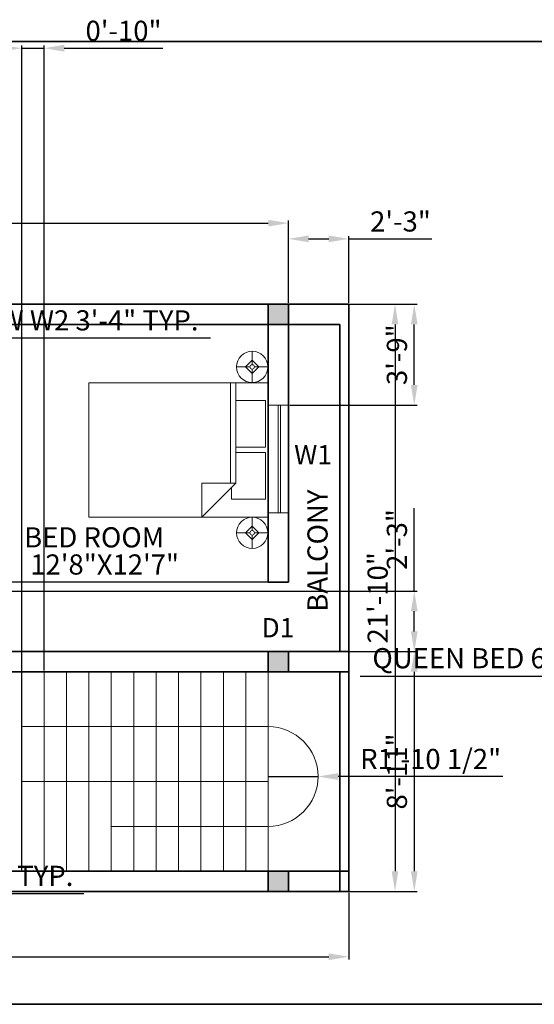
# Model space of a CAD drawing. Units: inches. Extents: x -281 to 2337, y 1647 to 2113.
# Tile 3 of 6: x 1459 to 1688, y 1674 to 2113. Entities that reach past the tile are written whole.
import ezdxf

# ---------------------------------------------------------------- set-up
doc = ezdxf.new("R2010")
doc.units = ezdxf.units.IN
for name, color, linetype, lineweight in [('A-ANNO-DIMS', 242, 'Continuous', 18), ('A-ANNO-IDEN', 11, 'Continuous', 18), ('A-ANNO-TTLB', 7, 'Continuous', 35), ('A-AREA-IDEN', 7, 'Continuous', 18), ('A-COLS', 1, 'Continuous', 35), ('A-FLOR-STRS', 7, 'Continuous', 18), ('A-FURN', 8, 'Continuous', 18), ('A-GLAZ', 3, 'Continuous', 18), ('A-WALL', 7, 'Continuous', 35)]:
    doc.layers.add(name, color=color, linetype=linetype, lineweight=lineweight)
doc.styles.get("Standard").update_dxf_attribs({"font": 'arial.ttf'})
doc.dimstyles.new('ISO-25', dxfattribs={"dimtxt": 9, "dimasz": 9, "dimexe": 1.25, "dimexo": 0.625, "dimgap": 2, "dimtad": 1, "dimdec": 1, "dimlunit": 4, "dimtxsty": 'Standard', "dimcen": 2.5, "dimadec": 0, "dimazin": 0, "dimtfac": 1, "dimtdec": 1, "dimtmove": 0, "dimatfit": 3, "dimfxl": 1, "dimarcsym": 0})

# ---------------------------------------------------------------- blocks, each defined once
blk = doc.blocks.new('Bed - Queen')
for p, q in [((0, -80.00003), (0, 0)), ((0, 0), (59.99999, 0)), ((59.99999, 0), (59.99999, -80.00003)), ((7.99999, -1.2), (28.79998, -1.2)), ((7.99999, -14.4), (7.99999, -1.2)), ((28.79998, -1.2), (28.79998, -14.4)), ((31.19999, -1.2), (51.99999, -1.2)), ((31.19999, -14.4), (31.19999, -1.2)), ((51.99999, -1.2), (51.99999, -16.4)), ((0, -14.4), (44.8, -14.4)), ((44.8, -16.8), (0, -16.8)), ((59.99999, -29.6), (44.8, -14.4)), ((44.8, -14.4), (44.8, -29.6)), ((51.99999, -16.4), (46.79936, -16.4)), ((44.8, -29.6), (59.99999, -29.6)), ((59.99999, -80.00003), (0, -80.00003))]:
    blk.add_line(p, q)
blk = doc.blocks.new('Lamp - Table')
for p, q in [((0, 7), (0, 1)), ((-1, 0), (-7, 0)), ((0, 3), (-3, 0)), ((-3, 0), (0, -3)), ((3, 0), (0, 3)), ((0, -3), (3, 0)), ((1, 0), (7, 0)), ((0, -1), (0, -7))]:
    blk.add_line(p, q)
for radius in [7, 1]:
    blk.add_circle((0, 0), radius)
blk = doc.blocks.new('*D8')
at = {"layer": 'A-ANNO-DIMS', "color": 0, "lineweight": -2, "transparency": 16777216}
for p, q in [((1084.42, 1986.77), (1084.42, 2023.6)), ((1093.42, 2022.35), (1569.42, 2022.35)), ((1578.42, 1986.77), (1578.42, 2023.6))]:
    blk.add_line(p, q, dxfattribs=at)
at = {"layer": 'A-ANNO-DIMS', "color": 0, "transparency": 16777216}
for points in [[(1093.42, 2023.85), (1093.42, 2020.85), (1084.42, 2022.35)], [(1569.42, 2023.85), (1569.42, 2020.85), (1578.42, 2022.35)]]:
    blk.add_solid(points, dxfattribs=at)
at = {"layer": 'Defpoints', "color": 0, "transparency": 16777216}
for p in [(1578.42, 2022.35), (1084.42, 1986.15), (1578.42, 1986.15)]:
    blk.add_point(p, dxfattribs=at)
at = {"layer": 'A-ANNO-DIMS', "color": 0, "transparency": 16777216, "insert": (1331.42, 2028.86), "char_height": 9, "attachment_point": 5}
blk.add_mtext('41\'-2"', dxfattribs=at)
blk = doc.blocks.new('*D9')
at = {"layer": 'A-ANNO-DIMS', "color": 0, "lineweight": -2, "transparency": 16777216}
for p, q in [((1579.05, 1986.15), (1627.28, 1986.15)), ((1626.03, 1977.15), (1626.03, 1733.15)), ((1579.05, 1724.15), (1627.28, 1724.15))]:
    blk.add_line(p, q, dxfattribs=at)
at = {"layer": 'A-ANNO-DIMS', "color": 0, "transparency": 16777216}
for points in [[(1624.53, 1977.15), (1627.53, 1977.15), (1626.03, 1986.15)], [(1624.53, 1733.15), (1627.53, 1733.15), (1626.03, 1724.15)]]:
    blk.add_solid(points, dxfattribs=at)
at = {"layer": 'Defpoints', "color": 0, "transparency": 16777216}
for p in [(1578.42, 1986.15), (1578.42, 1724.15), (1626.03, 1724.15)]:
    blk.add_point(p, dxfattribs=at)
at = {"layer": 'A-ANNO-DIMS', "color": 0, "transparency": 16777216, "insert": (1619.44, 1855.15), "char_height": 9, "attachment_point": 5, "rotation": 90}
blk.add_mtext('21\'-10"', dxfattribs=at)
blk = doc.blocks.new('COL-9x9')
h = blk.add_hatch(color=256)
h.dxf.hatch_style = 1
h.paths.add_polyline_path([(9, 9), (0, 9), (0, 0), (9, 0)])
for p, q in [((0, 9), (9, 9)), ((0, 0), (0, 9)), ((9, 9), (9, 0)), ((9, 0), (0, 0))]:
    blk.add_line(p, q)
blk = doc.blocks.new('WIN-W1-48')
for p, q in [((0, 48), (9, 48)), ((3.5, 0), (3.5, 48)), ((4.5, 0), (4.5, 48)), ((0, 0), (9, 0))]:
    blk.add_line(p, q)
blk = doc.blocks.new('*D21')
at = {"layer": 'A-ANNO-DIMS', "color": 0, "lineweight": -2, "transparency": 16777216}
for p, q in [((1354.42, 1976.52), (1354.42, 1969.9)), ((1394.42, 1976.52), (1394.42, 1969.9)), ((1363.42, 1971.15), (1385.42, 1971.15)), ((1394.42, 1971.15), (1543.66, 1971.15))]:
    blk.add_line(p, q, dxfattribs=at)
at = {"layer": 'A-ANNO-DIMS', "color": 0, "transparency": 16777216}
for points in [[(1363.42, 1972.65), (1363.42, 1969.65), (1354.42, 1971.15)], [(1385.42, 1972.65), (1385.42, 1969.65), (1394.42, 1971.15)]]:
    blk.add_solid(points, dxfattribs=at)
at = {"layer": 'Defpoints', "color": 0, "transparency": 16777216}
for p in [(1354.42, 1977.15), (1394.42, 1977.15), (1394.42, 1971.15)]:
    blk.add_point(p, dxfattribs=at)
at = {"layer": 'A-ANNO-DIMS', "color": 0, "transparency": 16777216, "insert": (1473.54, 1977.81), "char_height": 9, "attachment_point": 5}
blk.add_mtext('WINDOW W2 3\'-4" TYP.', dxfattribs=at)
blk = doc.blocks.new('*D25')
at = {"layer": 'A-ANNO-DIMS', "color": 0, "lineweight": -2, "transparency": 16777216}
for p, q in [((1755.88, 1820.1), (1610.49, 1820.1)), ((1755.88, 1808.73), (1755.88, 1821.35)), ((1826.88, 1820.1), (1764.88, 1820.1)), ((1835.88, 1808.73), (1835.88, 1821.35))]:
    blk.add_line(p, q, dxfattribs=at)
at = {"layer": 'A-ANNO-DIMS', "color": 0, "transparency": 16777216}
for points in [[(1764.88, 1821.6), (1764.88, 1818.6), (1755.88, 1820.1)], [(1826.88, 1821.6), (1826.88, 1818.6), (1835.88, 1820.1)]]:
    blk.add_solid(points, dxfattribs=at)
at = {"layer": 'Defpoints', "color": 0, "transparency": 16777216}
for p in [(1755.88, 1820.1), (1755.88, 1808.1), (1835.88, 1808.1)]:
    blk.add_point(p, dxfattribs=at)
at = {"layer": 'A-ANNO-DIMS', "color": 0, "transparency": 16777216, "insert": (1678.68, 1827.03), "char_height": 9, "attachment_point": 5}
blk.add_mtext('QUEEN BED 6\'-8" TYP.', dxfattribs=at)
blk = doc.blocks.new('*D29')
at = {"layer": 'A-ANNO-DIMS', "color": 0, "lineweight": -2, "transparency": 16777216}
for p, q in [((1254.1, 1733.03), (1254.1, 1722.01)), ((1323.39, 1733.03), (1323.39, 1722.01)), ((1263.1, 1723.26), (1314.39, 1723.26)), ((1323.39, 1723.26), (1487.21, 1723.26))]:
    blk.add_line(p, q, dxfattribs=at)
at = {"layer": 'A-ANNO-DIMS', "color": 0, "transparency": 16777216}
for points in [[(1263.1, 1724.76), (1263.1, 1721.76), (1254.1, 1723.26)], [(1314.39, 1724.76), (1314.39, 1721.76), (1323.39, 1723.26)]]:
    blk.add_solid(points, dxfattribs=at)
at = {"layer": 'Defpoints', "color": 0, "transparency": 16777216}
for p in [(1254.1, 1733.65), (1323.39, 1733.65), (1323.39, 1723.26)]:
    blk.add_point(p, dxfattribs=at)
at = {"layer": 'A-ANNO-DIMS', "color": 0, "transparency": 16777216, "insert": (1409.8, 1729.91), "char_height": 9, "attachment_point": 5}
blk.add_mtext('DINING SET 5\'-9 1/2" TYP.', dxfattribs=at)
blk = doc.blocks.new('*D42')
at = {"layer": 'A-ANNO-DIMS', "color": 0, "lineweight": -2, "transparency": 16777216}
for p, q in [((1084.42, 1723.52), (1084.42, 1693.7)), ((1605.42, 1723.52), (1605.42, 1693.7)), ((1093.42, 1694.95), (1596.42, 1694.95))]:
    blk.add_line(p, q, dxfattribs=at)
at = {"layer": 'A-ANNO-DIMS', "color": 0, "transparency": 16777216}
for points in [[(1093.42, 1696.45), (1093.42, 1693.45), (1084.42, 1694.95)], [(1596.42, 1696.45), (1596.42, 1693.45), (1605.42, 1694.95)]]:
    blk.add_solid(points, dxfattribs=at)
at = {"layer": 'Defpoints', "color": 0, "transparency": 16777216}
for p in [(1084.42, 1724.15), (1605.42, 1724.15), (1605.42, 1694.95)]:
    blk.add_point(p, dxfattribs=at)
at = {"layer": 'A-ANNO-DIMS', "color": 0, "transparency": 16777216, "insert": (1344.92, 1701.55), "char_height": 9, "attachment_point": 5}
blk.add_mtext('43\'-5"', dxfattribs=at)
blk = doc.blocks.new('*D44')
at = {"layer": 'A-ANNO-DIMS', "color": 0, "lineweight": -2, "transparency": 16777216}
for p, q in [((1606.05, 1831.15), (1635.87, 1831.15)), ((1634.62, 1822.15), (1634.62, 1733.15)), ((1606.05, 1724.15), (1635.87, 1724.15))]:
    blk.add_line(p, q, dxfattribs=at)
at = {"layer": 'A-ANNO-DIMS', "color": 0, "transparency": 16777216}
for points in [[(1633.12, 1822.15), (1636.12, 1822.15), (1634.62, 1831.15)], [(1633.12, 1733.15), (1636.12, 1733.15), (1634.62, 1724.15)]]:
    blk.add_solid(points, dxfattribs=at)
at = {"layer": 'Defpoints', "color": 0, "transparency": 16777216}
for p in [(1605.42, 1831.15), (1605.42, 1724.15), (1634.62, 1724.15)]:
    blk.add_point(p, dxfattribs=at)
at = {"layer": 'A-ANNO-DIMS', "color": 0, "transparency": 16777216, "insert": (1628.03, 1777.65), "char_height": 9, "attachment_point": 5, "rotation": 90}
blk.add_mtext('8\'-11"', dxfattribs=at)
blk = doc.blocks.new('*D48')
at = {"layer": 'A-ANNO-DIMS', "color": 0, "lineweight": -2, "transparency": 16777216}
for p, q in [((1579.05, 1986.15), (1635.87, 1986.15)), ((1634.62, 1950.15), (1634.62, 1977.15)), ((1579.05, 1941.15), (1635.87, 1941.15))]:
    blk.add_line(p, q, dxfattribs=at)
at = {"layer": 'A-ANNO-DIMS', "color": 0, "transparency": 16777216}
for points in [[(1633.12, 1977.15), (1636.12, 1977.15), (1634.62, 1986.15)], [(1633.12, 1950.15), (1636.12, 1950.15), (1634.62, 1941.15)]]:
    blk.add_solid(points, dxfattribs=at)
at = {"layer": 'Defpoints', "color": 0, "transparency": 16777216}
for p in [(1578.42, 1986.15), (1634.62, 1986.15), (1578.42, 1941.15)]:
    blk.add_point(p, dxfattribs=at)
at = {"layer": 'A-ANNO-DIMS', "color": 0, "transparency": 16777216, "insert": (1628.03, 1963.65), "char_height": 9, "attachment_point": 5, "rotation": 90}
blk.add_mtext('3\'-9"', dxfattribs=at)
blk = doc.blocks.new('*D57')
at = {"layer": 'A-ANNO-DIMS', "color": 0, "lineweight": -2, "transparency": 16777216}
for p, q in [((1577.8, 1862.15), (1053.97, 1862.15)), ((1055.22, 1840.15), (1055.22, 1853.15)), ((1577.8, 1831.15), (1053.97, 1831.15))]:
    blk.add_line(p, q, dxfattribs=at)
at = {"layer": 'A-ANNO-DIMS', "color": 0, "transparency": 16777216}
for points in [[(1053.72, 1853.15), (1056.72, 1853.15), (1055.22, 1862.15)], [(1053.72, 1840.15), (1056.72, 1840.15), (1055.22, 1831.15)]]:
    blk.add_solid(points, dxfattribs=at)
at = {"layer": 'Defpoints', "color": 0, "transparency": 16777216}
for p in [(1055.22, 1862.15), (1578.42, 1862.15), (1578.42, 1831.15)]:
    blk.add_point(p, dxfattribs=at)
at = {"layer": 'A-ANNO-DIMS', "color": 0, "transparency": 16777216, "insert": (1048.71, 1846.65), "char_height": 9, "attachment_point": 5, "rotation": 90}
blk.add_mtext('2\'-7"', dxfattribs=at)
blk = doc.blocks.new('*D58')
at = {"layer": 'A-ANNO-DIMS', "color": 0, "lineweight": -2, "transparency": 16777216}
for p, q in [((1634.62, 1858.15), (1634.62, 1895.23)), ((1418.05, 1858.15), (1635.87, 1858.15)), ((1634.62, 1840.15), (1634.62, 1849.15)), ((1418.05, 1831.15), (1635.87, 1831.15))]:
    blk.add_line(p, q, dxfattribs=at)
at = {"layer": 'A-ANNO-DIMS', "color": 0, "transparency": 16777216}
for points in [[(1633.12, 1849.15), (1636.12, 1849.15), (1634.62, 1858.15)], [(1633.12, 1840.15), (1636.12, 1840.15), (1634.62, 1831.15)]]:
    blk.add_solid(points, dxfattribs=at)
at = {"layer": 'Defpoints', "color": 0, "transparency": 16777216}
for p in [(1417.42, 1858.15), (1634.62, 1858.15), (1417.42, 1831.15)]:
    blk.add_point(p, dxfattribs=at)
at = {"layer": 'A-ANNO-DIMS', "color": 0, "transparency": 16777216, "insert": (1628.03, 1881.19), "char_height": 9, "attachment_point": 5, "rotation": 90}
blk.add_mtext('2\'-3"', dxfattribs=at)
blk = doc.blocks.new('*D59')
at = {"layer": 'A-ANNO-DIMS', "color": 0, "lineweight": -2, "transparency": 16777216}
for p, q in [((1578.42, 1986.77), (1578.42, 2016.6)), ((1587.42, 2015.35), (1596.42, 2015.35)), ((1605.42, 1986.77), (1605.42, 2016.6)), ((1605.42, 2015.35), (1642.5, 2015.35))]:
    blk.add_line(p, q, dxfattribs=at)
at = {"layer": 'A-ANNO-DIMS', "color": 0, "transparency": 16777216}
for points in [[(1587.42, 2016.85), (1587.42, 2013.85), (1578.42, 2015.35)], [(1596.42, 2016.85), (1596.42, 2013.85), (1605.42, 2015.35)]]:
    blk.add_solid(points, dxfattribs=at)
at = {"layer": 'Defpoints', "color": 0, "transparency": 16777216}
for p in [(1605.42, 2015.35), (1578.42, 1986.15), (1605.42, 1986.15)]:
    blk.add_point(p, dxfattribs=at)
at = {"layer": 'A-ANNO-DIMS', "color": 0, "transparency": 16777216, "insert": (1628.46, 2021.95), "char_height": 9, "attachment_point": 5}
blk.add_mtext('2\'-3"', dxfattribs=at)
blk = doc.blocks.new('*D60')
at = {"layer": 'A-ANNO-DIMS', "color": 0, "lineweight": -2, "transparency": 16777216}
for p, q in [((1417.42, 1733.77), (1417.42, 2101.68)), ((1459.42, 1733.77), (1459.42, 2101.68)), ((1426.42, 2100.43), (1450.42, 2100.43))]:
    blk.add_line(p, q, dxfattribs=at)
at = {"layer": 'A-ANNO-DIMS', "color": 0, "transparency": 16777216}
for points in [[(1426.42, 2101.93), (1426.42, 2098.93), (1417.42, 2100.43)], [(1450.42, 2101.93), (1450.42, 2098.93), (1459.42, 2100.43)]]:
    blk.add_solid(points, dxfattribs=at)
at = {"layer": 'Defpoints', "color": 0, "transparency": 16777216}
for p in [(1459.42, 2100.43), (1417.42, 1733.15), (1459.42, 1733.15)]:
    blk.add_point(p, dxfattribs=at)
at = {"layer": 'A-ANNO-DIMS', "color": 0, "transparency": 16777216, "insert": (1438.42, 2107.03), "char_height": 9, "attachment_point": 5}
blk.add_mtext('3\'-6"', dxfattribs=at)
blk = doc.blocks.new('*D61')
at = {"layer": 'A-ANNO-DIMS', "color": 0, "lineweight": -2, "transparency": 16777216}
for p, q in [((1459.42, 1822.77), (1459.42, 2101.68)), ((1469.42, 1822.77), (1469.42, 2101.68)), ((1450.42, 2100.43), (1441.42, 2100.43)), ((1459.42, 2100.43), (1469.42, 2100.43)), ((1478.42, 2100.43), (1522.34, 2100.43))]:
    blk.add_line(p, q, dxfattribs=at)
at = {"layer": 'A-ANNO-DIMS', "color": 0, "transparency": 16777216}
for points in [[(1450.42, 2101.93), (1450.42, 2098.93), (1459.42, 2100.43)], [(1478.42, 2101.93), (1478.42, 2098.93), (1469.42, 2100.43)]]:
    blk.add_solid(points, dxfattribs=at)
at = {"layer": 'Defpoints', "color": 0, "transparency": 16777216}
for p in [(1469.42, 2100.43), (1459.42, 1822.15), (1469.42, 1822.15)]:
    blk.add_point(p, dxfattribs=at)
at = {"layer": 'A-ANNO-DIMS', "color": 0, "transparency": 16777216, "insert": (1504.88, 2107.03), "char_height": 9, "attachment_point": 5}
blk.add_mtext('0\'-10"', dxfattribs=at)
blk = doc.blocks.new('*D70')
at = {"layer": 'A-ANNO-DIMS', "color": 0, "lineweight": -2, "transparency": 16777216}
for p, q in [((1569.42, 1775.4), (1591.67, 1775.4)), ((1674.18, 1775.4), (1600.67, 1775.4))]:
    blk.add_line(p, q, dxfattribs=at)
at = {"layer": 'A-ANNO-DIMS', "color": 0, "transparency": 16777216}
blk.add_solid([(1600.67, 1776.9), (1600.67, 1773.9), (1591.67, 1775.4)], dxfattribs=at)
at = {"layer": 'Defpoints', "color": 0, "transparency": 16777216}
for p in [(1569.42, 1775.4), (1591.67, 1775.4)]:
    blk.add_point(p, dxfattribs=at)
at = {"layer": 'A-ANNO-DIMS', "color": 0, "transparency": 16777216, "insert": (1641.93, 1782.05), "char_height": 9, "attachment_point": 5, "rotation": 0.0003}
blk.add_mtext('R1\'-10 1/2"', dxfattribs=at)

msp = doc.modelspace()

# ---------------------------------------------------------------- linework, layer by layer
at = {"layer": 'A-ANNO-TTLB'}
msp.add_lwpolyline([(1037.79, 2103.48), (2323.1, 2103.48), (2323.1, 1673.73), (1037.79, 1673.73)], close=True, dxfattribs=at)
at = {"layer": 'A-FLOR-STRS'}
for p, q in [((1459.42, 1822.15), (1459.42, 1733.15)), ((1469.42, 1822.15), (1469.42, 1733.15)), ((1479.42, 1822.15), (1479.42, 1733.15)), ((1489.42, 1822.15), (1489.42, 1733.15)), ((1499.42, 1822.15), (1499.42, 1733.15)), ((1509.42, 1822.15), (1509.42, 1733.15)), ((1519.42, 1822.15), (1519.42, 1733.15)), ((1529.42, 1822.15), (1529.42, 1733.15)), ((1539.42, 1822.15), (1539.42, 1733.15)), ((1549.42, 1822.15), (1549.42, 1733.15)), ((1559.42, 1822.15), (1559.42, 1753.15)), ((1569.42, 1822.15), (1569.42, 1724.15)), ((1569.42, 1797.65), (1459.42, 1797.65)), ((1549.42, 1773.15), (1459.42, 1773.15)), ((1569.42, 1773.15), (1549.42, 1773.15)), ((1569.42, 1753.15), (1499.42, 1753.15)), ((1559.42, 1753.15), (1559.42, 1733.15))]:
    msp.add_line(p, q, dxfattribs=at)
msp.add_arc((1569.42, 1775.4), 22.25, 270, 90, dxfattribs=at)
at = {"layer": 'A-WALL'}
for p, q in [((1084.42, 1986.15), (1605.42, 1986.15)), ((1578.42, 1986.15), (1578.42, 1862.15)), ((1605.42, 1986.15), (1605.42, 1822.15)), ((1093.42, 1977.15), (1601.42, 1977.15)), ((1569.42, 1977.15), (1569.42, 1862.15)), ((1601.42, 1977.15), (1601.42, 1831.15)), ((1569.42, 1862.15), (1578.42, 1862.15)), ((1408.42, 1831.15), (1605.42, 1831.15)), ((1569.42, 1831.15), (1569.42, 1822.15)), ((1578.42, 1831.15), (1578.42, 1822.15)), ((1605.42, 1826.15), (1605.42, 1724.15)), ((1417.42, 1822.15), (1605.42, 1822.15)), ((1601.42, 1822.15), (1601.42, 1724.15)), ((1605.42, 1733.15), (1413.42, 1733.15)), ((1578.42, 1733.15), (1578.42, 1724.15)), ((1605.42, 1724.15), (1084.42, 1724.15))]:
    msp.add_line(p, q, dxfattribs=at)

# ---------------------------------------------------------------- block references
at = {"layer": 'A-COLS', "rotation": 180}
for p in [(1578.42, 1986.15), (1578.42, 1831.15), (1578.42, 1733.15)]:
    msp.add_blockref('COL-9x9', p, dxfattribs=at)
at = {"layer": 'A-FURN'}
for p in [(1562.29, 1958.2), (1562.29, 1884.13)]:
    msp.add_blockref('Lamp - Table', p, dxfattribs=at)
at = {"layer": 'A-FURN', "rotation": 270}
msp.add_blockref('Bed - Queen', (1569.4, 1951.15), dxfattribs=at)
at = {"layer": 'A-GLAZ', "rotation": 180}
msp.add_blockref('WIN-W1-48', (1578.42, 1941.15), dxfattribs=at)

# ---------------------------------------------------------------- texts
at = {"layer": 'A-ANNO-IDEN'}
for s, p in [('W1', (1581.02, 1914.71)), ('D1', (1566.47, 1837.48))]:
    msp.add_text(s, height=8.623, dxfattribs=at).set_placement(p)
at = {"layer": 'A-AREA-IDEN'}
msp.add_text('BALCONY', height=9, rotation=90, dxfattribs=at).set_placement((1595.94, 1848.93))
for s, p in [('BED ROOM', (1460.5, 1877.63)), (' 12\'8"X12\'7"', (1460.5, 1865.52))]:
    msp.add_text(s, height=9, dxfattribs=at).set_placement(p)

# ---------------------------------------------------------------- dimensions: what is measured, and where the dimension line sits
at = {"layer": 'A-ANNO-DIMS'}
for base, p1, p2, override, picture, middle in [((1459.42, 2100.43), (1417.42, 1733.15), (1459.42, 1733.15), {"dimdec": 1, "dimlfac": 1, "dimrnd": 0, "dimzin": 1, "dimdsep": 46, "dimlunit": 4, "dimfrac": 2}, '*D60', (1438.42, 2107.03)), ((1469.42, 2100.43), (1459.42, 1822.15), (1469.42, 1822.15), {"dimdec": 1, "dimlfac": 1, "dimrnd": 0, "dimzin": 1, "dimdsep": 46, "dimlunit": 4, "dimfrac": 2}, '*D61', (1504.88, 2107.03)), ((1578.42, 2022.35), (1084.42, 1986.15), (1578.42, 1986.15), {"dimclrd": 0, "dimclre": 0, "dimclrt": 0}, '*D8', (1331.42, 2028.86)), ((1605.42, 2015.35), (1578.42, 1986.15), (1605.42, 1986.15), {"dimdec": 1, "dimlfac": 1, "dimrnd": 0, "dimzin": 1, "dimdsep": 46, "dimlunit": 4, "dimfrac": 2}, '*D59', (1628.46, 2021.95)), ((1605.42, 1694.95), (1084.42, 1724.15), (1605.42, 1724.15), {"dimdec": 1, "dimlfac": 1, "dimrnd": 0, "dimzin": 1, "dimdsep": 46, "dimlunit": 4, "dimfrac": 2}, '*D42', (1344.92, 1701.55))]:
    dim = msp.add_linear_dim(base=base, p1=p1, p2=p2, dimstyle='ISO-25', override=override, dxfattribs=at)
    dim.commit()
    dim.dimension.update_dxf_attribs({"geometry": picture, "text_midpoint": middle})
for base, p1, p2, text, picture, middle in [((1394.42, 1971.15), (1354.42, 1977.15), (1394.42, 1977.15), 'WINDOW W2 <> TYP.', '*D21', (1473.54, 1977.81)), ((1323.39, 1723.26), (1254.1, 1733.65), (1323.39, 1733.65), 'DINING SET <> TYP.', '*D29', (1409.8, 1729.91))]:
    dim = msp.add_linear_dim(base=base, p1=p1, p2=p2, text=text, dimstyle='ISO-25', override={"dimdec": 1, "dimlfac": 1, "dimrnd": 0, "dimzin": 1, "dimdsep": 46, "dimlunit": 4, "dimfrac": 2}, dxfattribs=at)
    dim.commit()
    dim.dimension.update_dxf_attribs({"geometry": picture, "text_midpoint": middle})
for base, p1, p2, angle, override, picture, middle in [((1626.03, 1724.15), (1578.42, 1986.15), (1578.42, 1724.15), 90, {"dimclrd": 0, "dimclre": 0, "dimclrt": 0}, '*D9', (1619.44, 1855.15)), ((1634.62, 1986.15), (1578.42, 1941.15), (1578.42, 1986.15), 90, {"dimdec": 1, "dimlfac": 1, "dimrnd": 0, "dimzin": 1, "dimdsep": 46, "dimlunit": 4, "dimfrac": 2}, '*D48', (1628.03, 1963.65)), ((1634.62, 1858.15), (1417.42, 1831.15), (1417.42, 1858.15), 90, {"dimdec": 1, "dimlfac": 1, "dimrnd": 0, "dimzin": 1, "dimdsep": 46, "dimlunit": 4, "dimfrac": 2}, '*D58', (1628.03, 1881.19)), ((1055.22, 1862.15), (1578.42, 1831.15), (1578.42, 1862.15), 90, {"dimdec": 1, "dimlfac": 1, "dimrnd": 0, "dimzin": 1, "dimdsep": 46, "dimlunit": 4, "dimfrac": 2}, '*D57', (1048.71, 1846.65)), ((1634.62, 1724.15), (1605.42, 1831.15), (1605.42, 1724.15), 270, {"dimdec": 1, "dimlfac": 1, "dimrnd": 0, "dimzin": 1, "dimdsep": 46, "dimlunit": 4, "dimfrac": 2}, '*D44', (1628.03, 1777.65))]:
    dim = msp.add_linear_dim(base=base, p1=p1, p2=p2, angle=angle, dimstyle='ISO-25', override=override, dxfattribs=at)
    dim.commit()
    dim.dimension.update_dxf_attribs({"geometry": picture, "text_midpoint": middle})
dim = msp.add_linear_dim(base=(1755.88, 1820.1), p1=(1835.88, 1808.1), p2=(1755.88, 1808.1), angle=180, text='QUEEN BED <> TYP.', dimstyle='ISO-25', override={"dimdec": 1, "dimlfac": 1, "dimrnd": 0, "dimzin": 1, "dimdsep": 46, "dimlunit": 4, "dimfrac": 2}, dxfattribs=at)
dim.commit()
dim.dimension.update_dxf_attribs({"geometry": '*D25', "text_midpoint": (1678.68, 1827.03)})
dim = msp.add_radius_dim(center=(1569.424572, 1775.398871), mpoint=(1591.674572, 1775.399), dimstyle='ISO-25', override={"dimdec": 1, "dimlfac": 1, "dimrnd": 0, "dimzin": 1, "dimdsep": 46, "dimlunit": 4, "dimfrac": 2}, dxfattribs=at)
dim.commit()
dim.dimension.update_dxf_attribs({"geometry": '*D70', "text_midpoint": (1641.92521555, 1782.05277019)})

doc.saveas('drawing.dxf')
